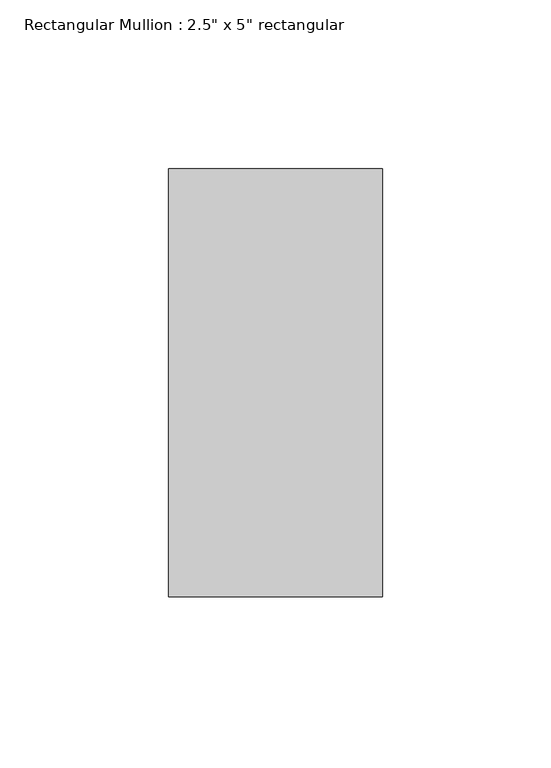
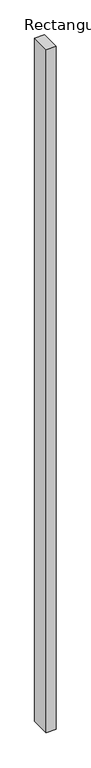
"""IFC4 building model written with IfcOpenShell, lengths in millimetres: member geometry."""

from ifc_helpers import new_model, si_unit, frame, origin, place, context, project, spatial, polyline, outline, extrude, source, transform, mapped, element, save


def member_67196db4(model_context):
    return source(origin(), model_context, "Body", "SweptSolid", [
        extrude(outline(polyline([(0.0, 63.5), (0.0, -63.5), (-63.5, -63.5), (-63.5, 63.5), (0.0, 63.5)])), frame((0.0, 0.0, -4630.6863081), z_axis=(0.0, 0.0, 1.0), x_axis=(1.0, 0.0, 0.0)), (0.0, 0.0, 1.0), 4630.6863081),
    ])


if __name__ == "__main__":
    model = new_model("IFC4")
    model_context = context("Model", 3, world=origin())
    ifc_project = project(units=[si_unit("LENGTHUNIT", "METRE", prefix="MILLI")], contexts=[model_context])
    site = spatial("IfcSite", under=ifc_project)
    building = spatial("IfcBuilding", under=site)
    placement = place(None, origin())
    member_shape = member_67196db4(model_context)
    element("IfcMember", 1, ObjectType="Rectangular Mullion : 2.5\" x 5\" rectangular", at=placement, inside=building, context=model_context, shape_type="MappedRepresentation", body=[
        mapped(member_shape, transform((0.0, 0.0, 0.0), x_axis=(1.0, 0.0, 0.0), y_axis=(0.0, 1.0, 0.0), z_axis=(0.0, 0.0, 1.0))),
    ])
    save(model, "model.ifc")

# Revit data of these elements
# Type "Rectangular Mullion : 2.5\" x 5\" rectangular"
#   built-in parameter 1007304 = 0.416667 (stored number, unit not read)
#   built-in parameter 1007301 = 0.104167 (stored number, unit not read)
#   built-in parameter 1007300 = 0.104167 (stored number, unit not read)
# Element 1 (IfcMember, "Rectangular Mullion : 2.5\" x 5\" rectangular")
#   Materials on its faces: "Aluminum"
# Materials
#   "Aluminum": class "Metal", colour RGB 247 247 247, transparency 0, Description = "Aluminum 6061", Cost = 0
